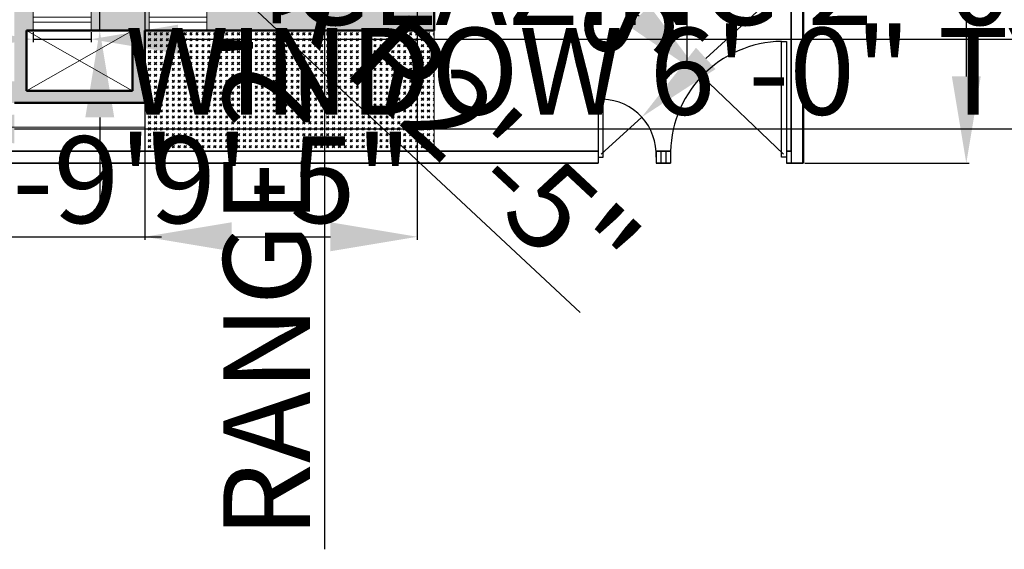
# Model space of a CAD drawing. Units: inches. Extents: x -299 to 1164, y -2 to 940.
# Tile 3 of 11: x 414 to 822, y -2 to 218. Entities that reach past the tile are written whole.
import ezdxf

# ---------------------------------------------------------------- set-up
doc = ezdxf.new("R2010")
doc.units = ezdxf.units.IN
for name, color, linetype, lineweight in [('A-FLOR-OPEN', 7, 'Continuous', 13), ('C-SITE-GATE', 20, 'Continuous', 25), ('C-SITE-PVMT', 7, 'Continuous', 18), ('C-SITE-WALL', 7, 'Continuous', 35), ('dimensions', 191, 'Continuous', 18), ('L-PLNT-PATT', 3, 'Continuous', 13), ('lawn', 3, 'Continuous', 18), ('outer walls', 7, 'Continuous', 50), ('windows', 130, 'Continuous', 18)]:
    doc.layers.add(name, color=color, linetype=linetype, lineweight=lineweight)
doc.layers.add('A-WALL-PATT', color=240, linetype='Continuous', lineweight=13, true_color=0xed1f24)
doc.styles.get("Standard").update_dxf_attribs({"font": 'arial.ttf'})
doc.dimstyles.new('ISO-25', dxfattribs={"dimtxt": 36, "dimasz": 36, "dimexe": 1.25, "dimexo": 0.625, "dimtad": 1, "dimlunit": 3, "dimtxsty": 'Standard', "dimcen": 2.5, "dimazin": 0, "dimtfac": 1, "dimtmove": 0, "dimatfit": 3, "dimfxl": 1, "dimarcsym": 0})

# ---------------------------------------------------------------- blocks, each defined once
blk = doc.blocks.new('glass')
at = {"layer": 'windows'}
for p, q in [((-12, 5.5), (-12, -3.5)), ((12, 5.5), (12, -3.5)), ((-12, 2), (12, 2)), ((-12, 0), (12, 0))]:
    blk.add_line(p, q, dxfattribs=at)
blk = doc.blocks.new('*D14')
at = {"layer": 'Defpoints', "color": 0, "transparency": 16777216}
for p in [(739.07, 638.49), (739.07, 158.49), (806.66, 158.49)]:
    blk.add_point(p, dxfattribs=at)
at = {"layer": 'dimensions', "color": 0, "lineweight": -2, "transparency": 16777216}
for p, q in [((739.7, 638.49), (807.91, 638.49)), ((806.66, 602.49), (806.66, 194.49)), ((739.7, 158.49), (807.91, 158.49))]:
    blk.add_line(p, q, dxfattribs=at)
at = {"layer": 'dimensions', "color": 0, "transparency": 16777216}
for points in [[(800.66, 602.49), (812.66, 602.49), (806.66, 638.49)], [(800.66, 194.49), (812.66, 194.49), (806.66, 158.49)]]:
    blk.add_solid(points, dxfattribs=at)
at = {"layer": 'dimensions', "color": 0, "transparency": 16777216, "insert": (787.65, 398.49), "char_height": 36, "attachment_point": 5, "rotation": 90}
blk.add_mtext("40'", dxfattribs=at)
blk = doc.blocks.new('*D23')
at = {"layer": 'Defpoints', "color": 0, "transparency": 16777216}
for p in [(701.12, 586.52), (690.74, 517.34), (701.12, 517.34)]:
    blk.add_point(p, dxfattribs=at)
at = {"layer": 'dimensions', "color": 0, "lineweight": -2, "transparency": 16777216}
for p, q in [((690.74, 622.52), (690.74, 658.52)), ((700.49, 586.52), (689.49, 586.52)), ((690.74, 586.52), (690.74, 517.34)), ((700.49, 517.34), (689.49, 517.34)), ((690.74, 481.34), (690.74, 197.66))]:
    blk.add_line(p, q, dxfattribs=at)
at = {"layer": 'dimensions', "color": 0, "transparency": 16777216}
for points in [[(684.74, 622.52), (696.74, 622.52), (690.74, 586.52)], [(684.74, 481.34), (696.74, 481.34), (690.74, 517.34)]]:
    blk.add_solid(points, dxfattribs=at)
at = {"layer": 'dimensions', "color": 0, "transparency": 16777216, "insert": (671.49, 321.5), "char_height": 36, "attachment_point": 5, "rotation": 90}
blk.add_mtext('SOFA 5\'-9"', dxfattribs=at)
blk = doc.blocks.new('*D29')
at = {"layer": 'Defpoints', "color": 0, "transparency": 16777216}
for p in [(304.07, 183.49), (376.07, 183.49), (376.07, 172.69)]:
    blk.add_point(p, dxfattribs=at)
at = {"layer": 'dimensions', "color": 0, "lineweight": -2, "transparency": 16777216}
for p, q in [((304.07, 182.86), (304.07, 171.44)), ((376.07, 182.86), (376.07, 171.44)), ((268.07, 172.69), (232.07, 172.69)), ((304.07, 172.69), (376.07, 172.69)), ((412.07, 172.69), (904.87, 172.69))]:
    blk.add_line(p, q, dxfattribs=at)
at = {"layer": 'dimensions', "color": 0, "transparency": 16777216}
for points in [[(268.07, 178.69), (268.07, 166.69), (304.07, 172.69)], [(412.07, 178.69), (412.07, 166.69), (376.07, 172.69)]]:
    blk.add_solid(points, dxfattribs=at)
at = {"layer": 'dimensions', "color": 0, "transparency": 16777216, "insert": (676.47, 191.94), "char_height": 36, "attachment_point": 5}
blk.add_mtext('WINDOW 6\'-0" TYP.', dxfattribs=at)
blk = doc.blocks.new('*D30')
at = {"layer": 'Defpoints', "color": 0, "transparency": 16777216}
for p in [(376.07, 192.49), (386.87, 192.49), (376.07, 183.49)]:
    blk.add_point(p, dxfattribs=at)
at = {"layer": 'dimensions', "color": 0, "lineweight": -2, "transparency": 16777216}
for p, q in [((386.87, 228.49), (386.87, 485.18)), ((376.7, 192.49), (388.12, 192.49)), ((386.87, 183.49), (386.87, 192.49)), ((376.7, 183.49), (388.12, 183.49)), ((386.87, 147.49), (386.87, 111.49))]:
    blk.add_line(p, q, dxfattribs=at)
at = {"layer": 'dimensions', "color": 0, "transparency": 16777216}
for points in [[(380.87, 228.49), (392.87, 228.49), (386.87, 192.49)], [(380.87, 147.49), (392.87, 147.49), (386.87, 183.49)]]:
    blk.add_solid(points, dxfattribs=at)
at = {"layer": 'dimensions', "color": 0, "transparency": 16777216, "insert": (367.87, 374.83), "char_height": 36, "attachment_point": 5, "rotation": 90}
blk.add_mtext('0\'-9" TYP.', dxfattribs=at)
blk = doc.blocks.new('*D33')
at = {"layer": 'Defpoints', "color": 0, "transparency": 16777216}
for p in [(419.84, 213.49), (443.84, 213.49), (443.84, 209.89)]:
    blk.add_point(p, dxfattribs=at)
at = {"layer": 'dimensions', "color": 0, "lineweight": -2, "transparency": 16777216}
for p, q in [((419.84, 212.86), (419.84, 208.64)), ((443.84, 212.86), (443.84, 208.64)), ((383.84, 209.89), (347.84, 209.89)), ((419.84, 209.89), (443.84, 209.89)), ((479.84, 209.89), (970.68, 209.89))]:
    blk.add_line(p, q, dxfattribs=at)
at = {"layer": 'dimensions', "color": 0, "transparency": 16777216}
for points in [[(383.84, 215.89), (383.84, 203.89), (419.84, 209.89)], [(479.84, 215.89), (479.84, 203.89), (443.84, 209.89)]]:
    blk.add_solid(points, dxfattribs=at)
at = {"layer": 'dimensions', "color": 0, "transparency": 16777216, "insert": (743.26, 229.13), "char_height": 36, "attachment_point": 5}
blk.add_mtext('GLAZING 2\'-0" TYP.', dxfattribs=at)
blk = doc.blocks.new('*D34')
at = {"layer": 'Defpoints', "color": 0, "transparency": 16777216}
for p in [(443.84, 222.49), (447.44, 222.49), (443.84, 213.49)]:
    blk.add_point(p, dxfattribs=at)
at = {"layer": 'dimensions', "color": 0, "lineweight": -2, "transparency": 16777216}
for p, q in [((447.44, 258.49), (447.44, 515.18)), ((444.47, 222.49), (448.69, 222.49)), ((447.44, 213.49), (447.44, 222.49)), ((444.47, 213.49), (448.69, 213.49)), ((447.44, 177.49), (447.44, 141.49))]:
    blk.add_line(p, q, dxfattribs=at)
at = {"layer": 'dimensions', "color": 0, "transparency": 16777216}
for points in [[(441.44, 258.49), (453.44, 258.49), (447.44, 222.49)], [(441.44, 177.49), (453.44, 177.49), (447.44, 213.49)]]:
    blk.add_solid(points, dxfattribs=at)
at = {"layer": 'dimensions', "color": 0, "transparency": 16777216, "insert": (428.44, 404.83), "char_height": 36, "attachment_point": 5, "rotation": 90}
blk.add_mtext('0\'-9" TYP.', dxfattribs=at)
blk = doc.blocks.new('*D41')
at = {"layer": 'Defpoints', "color": 0, "transparency": 16777216}
for p in [(545.04, 388.33), (540.54, 358.33), (545.04, 358.33)]:
    blk.add_point(p, dxfattribs=at)
at = {"layer": 'dimensions', "color": 0, "lineweight": -2, "transparency": 16777216}
for p, q in [((540.54, 424.33), (540.54, 460.33)), ((544.41, 388.33), (539.29, 388.33)), ((540.54, 388.33), (540.54, 358.33)), ((544.41, 358.33), (539.29, 358.33)), ((540.54, 322.33), (540.54, -1.56))]:
    blk.add_line(p, q, dxfattribs=at)
at = {"layer": 'dimensions', "color": 0, "transparency": 16777216}
for points in [[(534.54, 424.33), (546.54, 424.33), (540.54, 388.33)], [(534.54, 322.33), (546.54, 322.33), (540.54, 358.33)]]:
    blk.add_solid(points, dxfattribs=at)
at = {"layer": 'dimensions', "color": 0, "transparency": 16777216, "insert": (521.3, 142.39), "char_height": 36, "attachment_point": 5, "rotation": 90}
blk.add_mtext('RANGE 2\'-6"', dxfattribs=at)
blk = doc.blocks.new('*D45')
at = {"layer": 'Defpoints', "color": 0, "transparency": 16777216}
for p in [(466.07, 222.49), (579.07, 222.49), (579.07, 127.99)]:
    blk.add_point(p, dxfattribs=at)
at = {"layer": 'dimensions', "color": 0, "lineweight": -2, "transparency": 16777216}
for p, q in [((466.07, 221.86), (466.07, 126.74)), ((579.07, 221.86), (579.07, 126.74)), ((502.07, 127.99), (543.07, 127.99))]:
    blk.add_line(p, q, dxfattribs=at)
at = {"layer": 'dimensions', "color": 0, "transparency": 16777216}
for points in [[(502.07, 133.99), (502.07, 121.99), (466.07, 127.99)], [(543.07, 133.99), (543.07, 121.99), (579.07, 127.99)]]:
    blk.add_solid(points, dxfattribs=at)
at = {"layer": 'dimensions', "color": 0, "transparency": 16777216, "insert": (522.57, 146.99), "char_height": 36, "attachment_point": 5}
blk.add_mtext('9\'-5"', dxfattribs=at)
blk = doc.blocks.new('*D49')
at = {"layer": 'Defpoints', "color": 0, "transparency": 16777216}
for p in [(259.07, 183.49), (304.07, 183.49), (304.07, 127.99)]:
    blk.add_point(p, dxfattribs=at)
at = {"layer": 'dimensions', "color": 0, "lineweight": -2, "transparency": 16777216}
for p, q in [((259.07, 182.86), (259.07, 126.74)), ((304.07, 182.86), (304.07, 126.74)), ((223.07, 127.99), (187.07, 127.99)), ((259.07, 127.99), (304.07, 127.99)), ((340.07, 127.99), (472.99, 127.99))]:
    blk.add_line(p, q, dxfattribs=at)
at = {"layer": 'dimensions', "color": 0, "transparency": 16777216}
for points in [[(223.07, 133.99), (223.07, 121.99), (259.07, 127.99)], [(340.07, 133.99), (340.07, 121.99), (304.07, 127.99)]]:
    blk.add_solid(points, dxfattribs=at)
at = {"layer": 'dimensions', "color": 0, "transparency": 16777216, "insert": (424.53, 147.01), "char_height": 36, "attachment_point": 5}
blk.add_mtext('3\'-9"', dxfattribs=at)
blk = doc.blocks.new('*D59')
at = {"layer": 'Defpoints', "color": 0, "transparency": 16777216}
for p in [(697.05, 194.59), (730.81, 162.24)]:
    blk.add_point(p, dxfattribs=at)
at = {"layer": 'dimensions', "color": 0, "lineweight": -2, "transparency": 16777216}
for p, q in [((530.01, 354.68), (671.06, 219.5)), ((730.81, 162.24), (697.05, 194.59))]:
    blk.add_line(p, q, dxfattribs=at)
at = {"layer": 'dimensions', "color": 0, "transparency": 16777216}
blk.add_solid([(675.21, 223.83), (666.91, 215.17), (697.05, 194.59)], dxfattribs=at)
at = {"layer": 'dimensions', "color": 0, "transparency": 16777216, "insert": (600.7, 313.27), "char_height": 36, "attachment_point": 5, "rotation": 316.2186}
blk.add_mtext('R3\'-11"', dxfattribs=at)
blk = doc.blocks.new('*D60')
at = {"layer": 'Defpoints', "color": 0, "transparency": 16777216}
for p in [(672.12, 177.62), (655.34, 162.24)]:
    blk.add_point(p, dxfattribs=at)
at = {"layer": 'dimensions', "color": 0, "lineweight": -2, "transparency": 16777216}
for p, q in [((842.68, 333.96), (698.66, 201.95)), ((655.34, 162.24), (672.12, 177.62))]:
    blk.add_line(p, q, dxfattribs=at)
at = {"layer": 'dimensions', "color": 0, "transparency": 16777216}
blk.add_solid([(694.61, 206.37), (702.71, 197.52), (672.12, 177.62)], dxfattribs=at)
at = {"layer": 'dimensions', "color": 0, "transparency": 16777216, "insert": (771.3, 293.9), "char_height": 36, "attachment_point": 5, "rotation": 42.5105}
blk.add_mtext('R1\'-11"', dxfattribs=at)
blk = doc.blocks.new('*D62')
at = {"layer": 'Defpoints', "color": 0, "transparency": 16777216}
for p in [(420.34, 307.74), (441.36, 288.12)]:
    blk.add_point(p, dxfattribs=at)
at = {"layer": 'dimensions', "color": 0, "lineweight": -2, "transparency": 16777216}
for p, q in [((420.34, 307.74), (441.36, 288.12)), ((646.59, 96.57), (467.68, 263.55))]:
    blk.add_line(p, q, dxfattribs=at)
at = {"layer": 'dimensions', "color": 0, "transparency": 16777216}
blk.add_solid([(471.78, 267.94), (463.59, 259.17), (441.36, 288.12)], dxfattribs=at)
at = {"layer": 'dimensions', "color": 0, "transparency": 16777216, "insert": (583.27, 181.68), "char_height": 36, "attachment_point": 5, "rotation": 316.9755}
blk.add_mtext('3X R2\'-5"', dxfattribs=at)

msp = doc.modelspace()

# ---------------------------------------------------------------- hatches: boundary and pattern name
at = {"layer": 'A-WALL-PATT'}
h = msp.add_hatch(color=256, dxfattribs=at)
h.dxf.hatch_style = 1
h.paths.add_polyline_path([(312.071, 460.489), (307.071, 460.489), (307.071, 432.489), (307.071, 427.489), (372.071, 427.489), (372.071, 375.489), (372.071, 370.489), (380.071, 370.489, -0.0217424), (380.071, 372.989), (380.071, 375.489), (377.071, 375.489), (377.071, 427.489), (417.071, 427.489), (417.071, 489.489), (412.071, 489.489), (412.071, 484.489), (412.071, 432.489), (312.071, 432.489)], flags=17)
h.paths.add_polyline_path([(340.071, 372.989, -0.0217424), (340.071, 375.489), (268.071, 375.489), (268.071, 427.489), (268.071, 432.489), (268.071, 484.489), (268.071, 489.489), (268.071, 629.489), (412.071, 629.489), (412.071, 527.563, -0.0185322), (414.571, 527.489), (417.071, 527.489), (417.071, 629.489), (581.071, 629.489), (581.071, 553.489), (586.071, 553.489), (586.071, 629.489), (730.071, 629.489), (730.071, 405.489), (713.071, 405.489), (713.071, 396.489), (739.071, 396.489), (739.071, 638.489), (259.071, 638.489), (259.071, 183.489), (304.071, 183.489), (304.071, 192.489), (268.071, 192.489), (268.071, 370.489), (340.071, 370.489)])
h.paths.add_polyline_path([(417.071, 188.489), (417.071, 213.489), (461.071, 213.489), (461.071, 188.489)], flags=16)
h.paths.add_polyline_path([(586.071, 313.578), (577.071, 313.578), (577.071, 311.489), (575.54, 311.489), (575.54, 302.489), (586.071, 302.489)], flags=16)
h.paths.add_polyline_path([(586.071, 405.489), (586.071, 481.489), (581.071, 481.489), (581.071, 432.489), (499.071, 432.489), (499.071, 427.489), (577.071, 427.489), (577.071, 385.578), (586.071, 385.578), (586.071, 396.489)], flags=17)
h.paths.add_polyline_path([(641.071, 405.489), (624.071, 405.489, -0.0333689), (624.071, 400.989), (624.071, 396.489), (641.071, 396.489)], flags=17)
h.paths.add_polyline_path([(491.866, 222.489), (491.866, 213.489), (586.071, 213.489), (586.071, 222.489)])
edge = h.paths.add_edge_path()
edge.add_line((467.866, 213.489), (467.866, 222.489))
edge.add_line((467.866, 222.489), (466.071, 222.489))
edge.add_line((466.071, 222.489), (466.071, 302.489))
edge.add_line((466.071, 302.489), (527.54, 302.489))
edge.add_line((527.54, 302.489), (527.54, 311.489))
edge.add_line((527.54, 311.489), (449.071, 311.489))
edge.add_line((449.071, 311.489), (449.071, 308.989))
edge.add_arc((420.339, 307.739), 28.759, -2.4911, 2.4911, ccw=False)
edge.add_line((449.071, 306.489), (461.071, 306.489))
edge.add_line((461.071, 306.489), (461.071, 222.489))
edge.add_line((461.071, 222.489), (443.844, 222.489))
edge.add_line((443.844, 222.489), (443.844, 213.489))
edge.add_line((443.844, 213.489), (419.844, 213.489))
edge.add_line((419.844, 213.489), (419.844, 222.489))
edge.add_line((419.844, 222.489), (417.071, 222.489))
edge.add_line((417.071, 222.489), (417.071, 306.489))
edge.add_line((417.071, 306.489), (417.071, 311.489))
edge.add_line((417.071, 311.489), (417.071, 375.489))
edge.add_line((417.071, 375.489), (412.071, 375.489))
edge.add_line((412.071, 375.489), (412.071, 370.489))
edge.add_line((412.071, 370.489), (412.071, 192.489))
edge.add_line((412.071, 192.489), (376.071, 192.489))
edge.add_line((376.071, 192.489), (376.071, 183.489))
edge.add_line((376.071, 183.489), (412.071, 183.489))
edge.add_line((412.071, 183.489), (466.071, 183.489))
edge.add_line((466.071, 183.489), (466.071, 213.489))
edge.add_line((466.071, 213.489), (467.866, 213.489))
at = {"layer": 'L-PLNT-PATT'}
h = msp.add_hatch(dxfattribs=at)
h.set_pattern_fill('GOST_GLASS', color=256, scale=0.29)
h.paths.add_polyline_path([(586.071, 213.489), (466.071, 213.489), (466.071, 183.489), (466.071, 163.489), (586.071, 163.489)])

# ---------------------------------------------------------------- linework, layer by layer
at = {"layer": 'A-FLOR-OPEN'}
for p, q in [((417.071, 213.489), (461.071, 188.489)), ((461.071, 213.489), (417.071, 188.489))]:
    msp.add_line(p, q, dxfattribs=at)
at = {"layer": 'C-SITE-GATE'}
for p, q in [((654.071, 163.489), (654.071, 158.489)), ((678.071, 163.489), (678.071, 158.489)), ((680.071, 163.489), (680.071, 158.489)), ((682.071, 163.489), (682.071, 158.489)), ((684.071, 163.489), (684.071, 158.489)), ((732.071, 163.489), (732.071, 158.489)), ((734.071, 163.489), (734.071, 158.489))]:
    msp.add_line(p, q, dxfattribs=at)
for points in [[(730.071, 208.989), (732.071, 208.989), (732.071, 160.989), (730.071, 160.989)], [(656.071, 184.989), (654.071, 184.989), (654.071, 160.989), (656.071, 160.989)]]:
    msp.add_lwpolyline(points, close=True, dxfattribs=at)
for centre, radius, start, end in [((730.81, 162.239), 46.756, 90.90579, 181.53196), ((655.344, 162.239), 22.762, 356.8519, 88.16899)]:
    msp.add_arc(centre, radius, start, end, dxfattribs=at)
at = {"layer": 'C-SITE-PVMT'}
msp.add_line((264.071, 173.489), (466.071, 173.489), dxfattribs=at)
at = {"layer": 'C-SITE-WALL'}
for p, q in [((734.071, 163.489), (734.071, 396.489)), ((264.071, 163.489), (654.071, 163.489)), ((678.071, 163.489), (684.071, 163.489)), ((732.071, 163.489), (734.071, 163.489)), ((259.071, 158.489), (654.071, 158.489)), ((678.071, 158.489), (684.071, 158.489)), ((732.071, 158.489), (739.071, 158.489))]:
    msp.add_line(p, q, dxfattribs=at)
at = {"layer": 'lawn'}
for p, q in [((586.071, 213.489), (586.071, 163.489)), ((466.071, 163.489), (466.071, 183.489))]:
    msp.add_line(p, q, dxfattribs=at)
at = {"layer": 'outer walls'}
for p, q in [((739.071, 158.489), (739.071, 638.489)), ((586.071, 222.489), (586.071, 213.489)), ((461.071, 213.489), (417.071, 213.489)), ((417.071, 213.489), (417.071, 188.489)), ((461.071, 213.489), (461.071, 188.489)), ((586.071, 213.489), (466.071, 213.489)), ((466.071, 213.489), (466.071, 183.489)), ((461.071, 188.489), (417.071, 188.489)), ((466.071, 183.489), (412.071, 183.489))]:
    msp.add_line(p, q, dxfattribs=at)

# ---------------------------------------------------------------- block references
at = {"layer": 'windows'}
for p in [(431.844, 216.989), (479.866, 216.989)]:
    msp.add_blockref('glass', p, dxfattribs=at)

# ---------------------------------------------------------------- dimensions: what is measured, and where the dimension line sits
at = {"layer": 'dimensions'}
for base, p1, p2, angle, text, picture, middle in [((690.742, 517.338), (701.119, 586.518), (701.119, 517.338), 270, 'SOFA <>', '*D23', (671.49, 321.5)), ((447.444, 222.489), (443.844, 213.489), (443.844, 222.489), 90, '<> TYP.', '*D34', (428.438, 404.833)), ((386.871, 192.489), (376.071, 183.489), (376.071, 192.489), 90, '<> TYP.', '*D30', (367.865, 374.833)), ((540.536, 358.335), (545.036, 388.335), (545.036, 358.335), 270, 'RANGE <>', '*D41', (521.297, 142.385))]:
    dim = msp.add_linear_dim(base=base, p1=p1, p2=p2, angle=angle, text=text, dimstyle='ISO-25', override={"dimdec": 1, "dimlfac": 1, "dimrnd": 0, "dimzin": 1, "dimdsep": 46, "dimlunit": 4, "dimfrac": 2}, dxfattribs=at)
    dim.commit()
    dim.dimension.update_dxf_attribs({"geometry": picture, "text_midpoint": middle})
dim = msp.add_linear_dim(base=(806.659, 158.489), p1=(739.071, 638.489), p2=(739.071, 158.489), angle=90, dimstyle='ISO-25', override={"dimclrd": 0, "dimclre": 0, "dimclrt": 0}, dxfattribs=at)
dim.commit()
dim.dimension.update_dxf_attribs({"geometry": '*D14', "text_midpoint": (787.654, 398.489)})
for center, mpoint, picture, middle in [((730.81, 162.239), (697.053, 194.59), '*D59', (600.698, 313.273)), ((655.344, 162.239), (672.123, 177.62), '*D60', (771.303, 293.901))]:
    dim = msp.add_radius_dim(center=center, mpoint=mpoint, dimstyle='ISO-25', override={"dimdec": 1, "dimlfac": 1, "dimrnd": 0, "dimzin": 1, "dimdsep": 46, "dimlunit": 4, "dimfrac": 2}, dxfattribs=at)
    dim.commit()
    dim.dimension.update_dxf_attribs({"geometry": picture, "text_midpoint": middle})
for base, p1, p2, text, picture, middle in [((443.844, 209.889), (419.844, 213.489), (443.844, 213.489), 'GLAZING <> TYP.', '*D33', (743.261, 229.128)), ((376.071, 172.689), (304.071, 183.489), (376.071, 183.489), 'WINDOW <> TYP.', '*D29', (676.471, 191.94))]:
    dim = msp.add_linear_dim(base=base, p1=p1, p2=p2, text=text, dimstyle='ISO-25', override={"dimdec": 1, "dimlfac": 1, "dimrnd": 0, "dimzin": 1, "dimdsep": 46, "dimlunit": 4, "dimfrac": 2}, dxfattribs=at)
    dim.commit()
    dim.dimension.update_dxf_attribs({"geometry": picture, "text_midpoint": middle})
dim = msp.add_radius_dim(center=(420.339, 307.739), mpoint=(441.364, 288.116), text='3X <>', dimstyle='ISO-25', override={"dimdec": 1, "dimlfac": 1, "dimrnd": 0, "dimzin": 1, "dimdsep": 46, "dimlunit": 4, "dimfrac": 2}, dxfattribs=at)
dim.commit()
dim.dimension.update_dxf_attribs({"geometry": '*D62', "text_midpoint": (583.273, 181.684)})
for base, p1, p2, picture, middle in [((579.071, 127.989), (466.071, 222.489), (579.071, 222.489), '*D45', (522.571, 146.995)), ((304.071, 127.989), (259.071, 183.489), (304.071, 183.489), '*D49', (424.532, 147.007))]:
    dim = msp.add_linear_dim(base=base, p1=p1, p2=p2, dimstyle='ISO-25', override={"dimdec": 1, "dimlfac": 1, "dimrnd": 0, "dimzin": 1, "dimdsep": 46, "dimlunit": 4, "dimfrac": 2}, dxfattribs=at)
    dim.commit()
    dim.dimension.update_dxf_attribs({"geometry": picture, "text_midpoint": middle})

doc.saveas('drawing.dxf')
